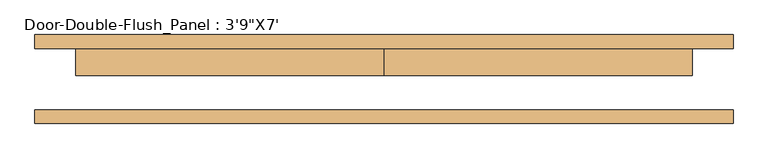
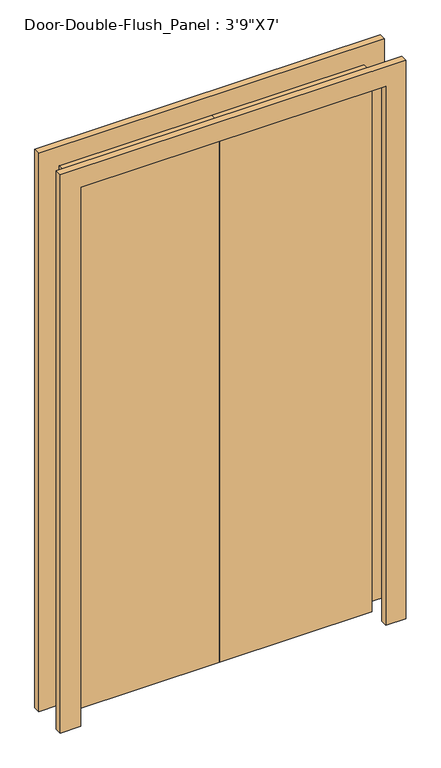
"""IFC4 building model written with IfcOpenShell, lengths in millimetres: door geometry."""

from ifc_helpers import new_model, si_unit, frame, origin, origin_with_axes, place, context, project, spatial, polyline, outline, extrude, source, transform, mapped, element, save


def door_31bd1cdd(model_context):
    return source(origin(), model_context, "Body", "SweptSolid", [
        extrude(outline(polyline([(2133.6, -571.5), (2133.6, 571.5), (0.0, 571.5), (0.0, 647.7), (2209.8, 647.7), (2209.8, -647.7), (0.0, -647.7), (0.0, -571.5), (2133.6, -571.5)])), frame((0.0, 57.15, 0.0), z_axis=(0.0, 1.0, 0.0), x_axis=(0.0, 0.0, 1.0)), (0.0, 0.0, 1.0), 25.4),
        extrude(outline(polyline([(2133.6, -571.5), (2133.6, 571.5), (0.0, 571.5), (0.0, 647.7), (2209.8, 647.7), (2209.8, -647.7), (0.0, -647.7), (0.0, -571.5), (2133.6, -571.5)])), frame((0.0, -82.55, 0.0), z_axis=(0.0, 1.0, 0.0), x_axis=(0.0, 0.0, 1.0)), (0.0, 0.0, 1.0), 25.4),
        extrude(outline(polyline([(-571.5, 57.15), (0.0, 57.15), (0.0, 6.35), (-571.5, 6.35), (-571.5, 57.15)])), origin_with_axes(), (0.0, 0.0, 1.0), 2133.6),
        extrude(outline(polyline([(0.0, 57.15), (571.5, 57.15), (571.5, 6.35), (0.0, 6.35), (0.0, 57.15)])), origin_with_axes(), (0.0, 0.0, 1.0), 2133.6),
    ])


if __name__ == "__main__":
    model = new_model("IFC4")
    model_context = context("Model", 3, world=origin())
    ifc_project = project(units=[si_unit("LENGTHUNIT", "METRE", prefix="MILLI")], contexts=[model_context])
    site = spatial("IfcSite", under=ifc_project)
    building = spatial("IfcBuilding", under=site)
    placement = place(None, origin())
    door_shape = door_31bd1cdd(model_context)
    element("IfcDoor", 1, ObjectType="Door-Double-Flush_Panel : 3'9\"X7'", at=placement, inside=building, context=model_context, shape_type="MappedRepresentation", body=[
        mapped(door_shape, transform((0.0, 0.0, 0.0), x_axis=(1.0, 0.0, 0.0), y_axis=(0.0, 1.0, 0.0), z_axis=(0.0, 0.0, 1.0))),
    ])
    save(model, "model.ifc")

# Revit data of these elements
# Type "Door-Double-Flush_Panel : 3'9\"X7'"
#   Type Mark = "11"
#   Construction Type Id = "DOOR"
#   Assembly Code = "C1020"
#   Analytic Construction = "Wooden"
#   Thickness = 0' - 2"
#   Thermal Resistance (R) = 2.5876 (h·ft²·°F)/BTU
#   Swing Angle [instance default] = 90.00°
#   Panel Width = 1' - 10 1/2"
#   Heat Transfer Coefficient (U) = 0.3865 BTU/(h·ft²·°F)
#   Height = 7' - 0"
#   Trim Projection Ext = 0' - 1"
#   Trim Projection Int = 0' - 1"
#   Trim Width = 0' - 3"
#   Width = 3' - 9"
#   Define Thermal Properties by = 1
#   Panel Material = Wood - Birch - Solid Stained Light Low Gloss
#   Trim Material = Paint - Sienna
#   Visual Light Transmittance = 0
#   Solar Heat Gain Coefficient = 0
#   Function = (empty or 0)
#   Wall Closure = (empty or 0)
# Element 1 (IfcDoor, "Door-Double-Flush_Panel : 3'9\"X7'")
#   Materials on its faces: "Paint - Sienna", "Wood - Birch - Solid Stained Light Low Gloss"
# Materials
#   "Wood - Birch - Solid Stained Light Low Gloss": class "Wood", colour RGB 210 159 95, transparency 0, Cost = 0
#   "Paint - Sienna": colour RGB 118 70 51, transparency 0, Cost = 0
